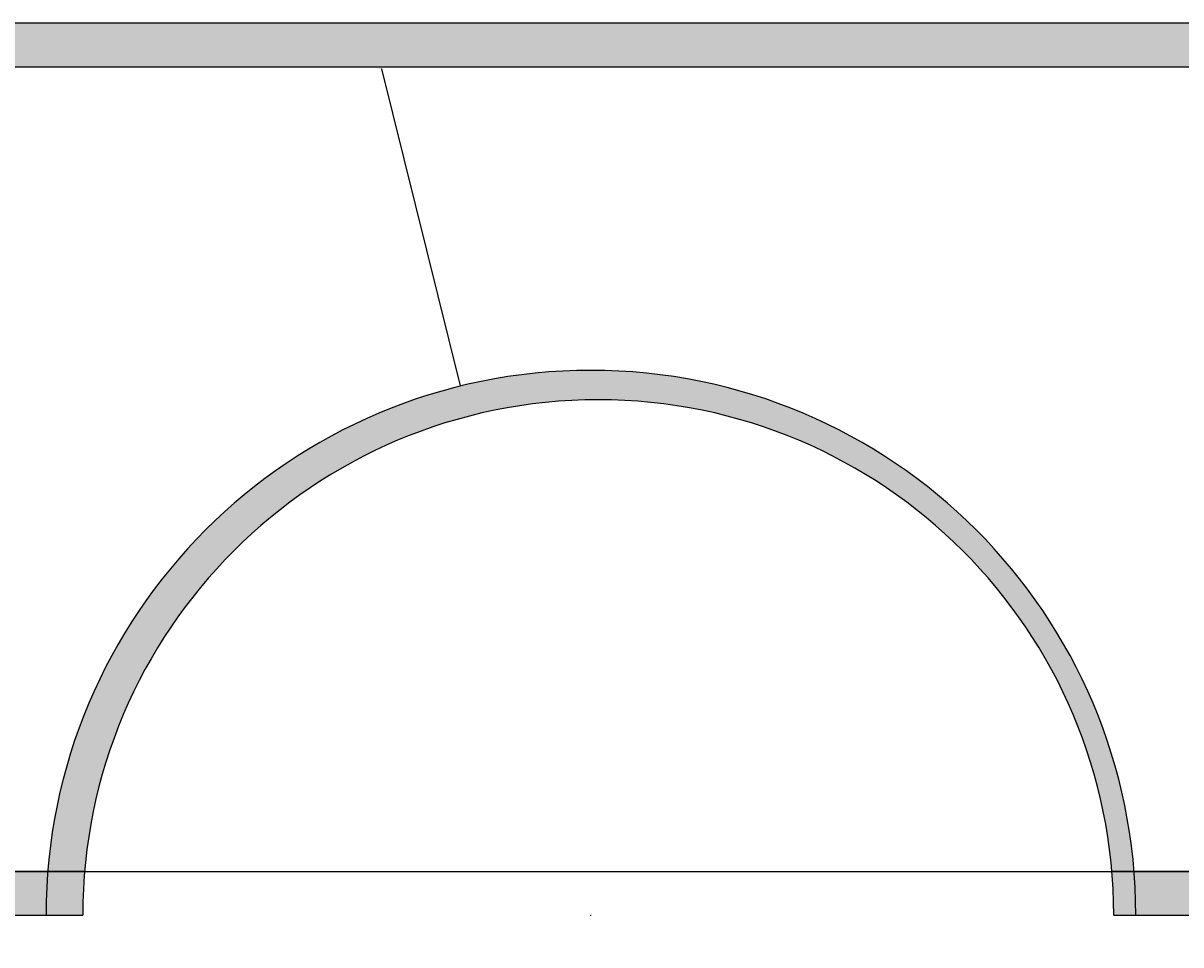
# Model space of a CAD drawing. Units: inches. Extents: x 35362 to 73946, y 43607 to 67532.
# Tile 133 of 134: x 69000 to 69530, y 45436 to 45858. Entities that reach past the tile are written whole.
import ezdxf

# ---------------------------------------------------------------- set-up
doc = ezdxf.new("R2010")
doc.units = ezdxf.units.IN
doc.header["$MEASUREMENT"] = 0
for name, color, linetype, lineweight in [('A-ANNO-DIMS', 2, 'Continuous', 18), ('E-SYMB', 1, 'Continuous', 25), ('E-SYMB-PATT', 1, 'Continuous', 13)]:
    doc.layers.add(name, color=color, linetype=linetype, lineweight=lineweight)
doc.styles.get("Standard").update_dxf_attribs({"font": 'arial.ttf'})
doc.dimstyles.get("Standard").update_dxf_attribs({"dimtxt": 0.18, "dimasz": 0.18, "dimexe": 0.18, "dimexo": 0.0625, "dimgap": 0.09, "dimtad": 0, "dimtih": 1, "dimtoh": 1, "dimdec": 4, "dimzin": 0, "dimdsep": 46, "dimtxsty": 'Standard', "dimcen": 0.09, "dimadec": 0, "dimazin": 0, "dimtfac": 1, "dimtdec": 4, "dimtofl": 0, "dimtmove": 0, "dimatfit": 3, "dimfxl": 1, "dimtolj": 1, "dimtzin": 0, "dimarcsym": 0})

# ---------------------------------------------------------------- blocks, each defined once
blk = doc.blocks.new('CT-CORE')
for p, q in [((270.6681283192447, 1387.996120092102), (270.6681283192447, -5.34733626409e-05)), ((290.6681283192447, -5.34733626409e-05), (290.6681283192593, 1387.996120092102)), ((658.9826659540267, 1387.996120092102), (658.9826659540267, 1014.585417332389)), ((678.9826659540413, 1015.434583844784), (678.9826659540413, 1387.996120092102)), ((658.9826659540267, 544.3844491987692), (658.9826659540267, -5.34733626409e-05)), ((678.9826659540267, -5.34733626409e-05), (678.9826659540413, 543.5352826863744))]:
    blk.add_line(p, q)
blk.add_arc((678.9826659540267, 779.4849332655793), 235.9496505792049, 90, 270)
blk = doc.blocks.new('*D5')
at = {"layer": 'A-ANNO-DIMS', "color": 0, "lineweight": -2, "transparency": 16777216}
for p, q in [((37121.949085, 46919.318283), (37121.949085, 43606.678996)), ((69871.496302, 45449.831951), (69871.496302, 43606.678996)), ((37122.129085, 43606.858996), (53496.2943647142, 43606.858996)), ((69871.316302, 43606.858996), (53497.15102228581, 43606.858996))]:
    blk.add_line(p, q, dxfattribs=at)
at = {"layer": 'A-ANNO-DIMS', "color": 0, "transparency": 16777216}
for points in [[(37122.129085, 43606.888996), (37122.129085, 43606.828996), (37121.949085, 43606.858996)], [(69871.316302, 43606.888996), (69871.316302, 43606.828996), (69871.496302, 43606.858996)]]:
    blk.add_solid(points, dxfattribs=at)
at = {"layer": 'Defpoints', "color": 0, "transparency": 16777216}
for p in [(37121.949085, 46919.380783), (69871.496302, 45449.894451), (69871.496302, 43606.858996)]:
    blk.add_point(p, dxfattribs=at)
at = {"layer": 'A-ANNO-DIMS', "color": 0, "transparency": 16777216, "insert": (53496.7226935, 43606.858996), "char_height": 0.18, "attachment_point": 5}
blk.add_mtext('\\A1;32750', dxfattribs=at)
blk = doc.blocks.new('*D24')
at = {"layer": 'A-ANNO-DIMS', "color": 0, "lineweight": -2, "transparency": 16777216}
for p, q in [((69163.64110083134, 45837.29257087316), (69163.82110083134, 45837.29257087316)), ((69163.82110083134, 45837.29257087316), (69199.7049619239, 45692.19301188657)), ((69259.53663199997, 45449.89445099998), (69259.71663199997, 45449.89445099998)), ((69259.62663199996, 45449.804451), (69259.62663199996, 45449.98445099999))]:
    blk.add_line(p, q, dxfattribs=at)
at = {"layer": 'A-ANNO-DIMS', "color": 0, "transparency": 16777216}
blk.add_solid([(69199.73408457165, 45692.20021406591), (69199.67583927614, 45692.18580970722), (69199.74817499997, 45692.018276)], dxfattribs=at)
at = {"layer": 'Defpoints', "color": 0, "transparency": 16777216}
for p in [(69199.74817499997, 45692.018276), (69259.62663199997, 45449.894451)]:
    blk.add_point(p, dxfattribs=at)
at = {"layer": 'A-ANNO-DIMS', "color": 0, "transparency": 16777216, "insert": (69162.9682495353, 45837.29257087316), "char_height": 0.18, "attachment_point": 5}
blk.add_mtext('\\A1;5X R249.4', dxfattribs=at)
blk = doc.blocks.new('*D75')
at = {"layer": 'A-ANNO-DIMS', "color": 0, "lineweight": -2, "transparency": 16777216}
for p, q in [((55181.69646300003, 45838.20898900001), (73945.82566600003, 45838.20898900001)), ((73945.64566600005, 45838.02898900001), (73945.64566600005, 45654.23368452933)), ((73945.64566600005, 45470.07445100001), (73945.64566600005, 45653.86975547068)), ((55181.69646300003, 45469.89445100001), (73945.82566600003, 45469.89445100001))]:
    blk.add_line(p, q, dxfattribs=at)
at = {"layer": 'A-ANNO-DIMS', "color": 0, "transparency": 16777216}
for points in [[(73945.61566600006, 45838.02898900001), (73945.67566600005, 45838.02898900001), (73945.64566600005, 45838.20898900001)], [(73945.61566600006, 45470.07445100001), (73945.67566600005, 45470.07445100001), (73945.64566600005, 45469.89445100001)]]:
    blk.add_solid(points, dxfattribs=at)
at = {"layer": 'Defpoints', "color": 0, "transparency": 16777216}
for p in [(55181.63396300002, 45838.20898900001), (55181.63396300002, 45469.89445100001), (73945.64566600005, 45469.89445100001)]:
    blk.add_point(p, dxfattribs=at)
at = {"layer": 'A-ANNO-DIMS', "color": 0, "transparency": 16777216, "insert": (73945.64566600005, 45654.05171999998), "char_height": 0.18, "attachment_point": 5}
blk.add_mtext('\\A1;368.3', dxfattribs=at)

msp = doc.modelspace()

# ---------------------------------------------------------------- hatches: boundary and pattern name
at = {"layer": 'E-SYMB-PATT'}
h = msp.add_hatch(color=256, dxfattribs=at)
h.dxf.hatch_style = 1
h.paths.add_polyline_path([(69871.49630189747, 45838.20898892413), (69871.49630189747, 45858.20898892414), (68483.50012833202, 45858.20898892414), (68483.50012833202, 45838.20898892414)])
h = msp.add_hatch(color=256, dxfattribs=at)
h.dxf.hatch_style = 1
h.paths.add_polyline_path([(69498.08559913776, 45469.89445128936), (69508.24154776601, 45469.89445128936, 0.3908929169039177), (69259.62663215057, 45699.3125265495, 0.3908929169039177), (69011.01171653513, 45469.89445128936), (69027.88463100414, 45469.89445128936, -0.389569854577291), (69262.98511507096, 45685.84410186857, -0.389569854577291)])
h = msp.add_hatch(color=256, dxfattribs=at)
h.dxf.hatch_style = 1
h.paths.add_polyline_path([(69027.03546449174, 45449.89445128935, -0.0212196039209565), (69027.88463100414, 45469.89445128936), (69011.01171653513, 45469.89445128936, 0.0200709024740955), (69010.20855689044, 45449.89445128935)])
h.paths.add_polyline_path([(69010.20855689044, 45449.89445128935, -0.0200709024740953), (69011.01171653513, 45469.89445128936), (68483.50012833202, 45469.89445128936), (68483.50012833202, 45449.89445128936)])
h.paths.add_polyline_path([(69871.49630189747, 45449.89445128935), (69871.49630189747, 45469.89445128936), (69508.24154776601, 45469.89445128936, -0.0200709024740959), (69509.04470741072, 45449.89445128935)])
h.paths.add_polyline_path([(69509.04470741072, 45449.89445128935, 0.020070902474096), (69508.24154776601, 45469.89445128936), (69498.08559913776, 45469.89445128936, -0.0212196039209564), (69498.93476565015, 45449.89445128935)])

# ---------------------------------------------------------------- linework, layer by layer
at = {"layer": 'E-SYMB'}
msp.add_arc((69259.62663215057, 45449.89445128936), 249.4180752601387, 0, 180, dxfattribs=at)

# ---------------------------------------------------------------- block references
at = {"layer": 'E-SYMB', "rotation": 269.9999999999974}
msp.add_blockref('CT-CORE', (68483.50018180539, 46128.87711724339), dxfattribs=at)

# ---------------------------------------------------------------- dimensions: what is measured, and where the dimension line sits
at = {"layer": 'A-ANNO-DIMS'}
dim = msp.add_linear_dim(base=(69871.496302, 43606.858996), p1=(37121.949085, 46919.380783), p2=(69871.496302, 45449.894451), dimstyle='Standard', override={"dimdec": 0, "dimlfac": 1, "dimrnd": 0, "dimzin": 0, "dimdsep": 46, "dimlunit": 2}, dxfattribs=at)
dim.commit()
dim.dimension.update_dxf_attribs({"geometry": '*D5', "text_midpoint": (53496.7226935, 43606.858996)})
dim = msp.add_linear_dim(base=(73945.64566600005, 45469.89445100001), p1=(55181.633963, 45838.20898899999), p2=(55181.633963, 45469.894451), angle=90, dimstyle='Standard', override={"dimdec": 1, "dimlfac": 1, "dimrnd": 0, "dimzin": 0, "dimdsep": 46, "dimlunit": 2}, dxfattribs=at)
dim.commit()
dim.dimension.update_dxf_attribs({"geometry": '*D75', "text_midpoint": (73945.64566600005, 45654.05171999998)})
dim = msp.add_radius_dim(center=(69259.62663199997, 45449.894451), mpoint=(69199.74817499997, 45692.018276), text='5X <>', dimstyle='Standard', override={"dimdec": 1, "dimlfac": 1, "dimrnd": 0, "dimzin": 0, "dimdsep": 46, "dimlunit": 2}, dxfattribs=at)
dim.commit()
dim.dimension.update_dxf_attribs({"geometry": '*D24', "text_midpoint": (69162.9682495353, 45837.29257087316), "dimtype": 164})

doc.saveas('drawing.dxf')
